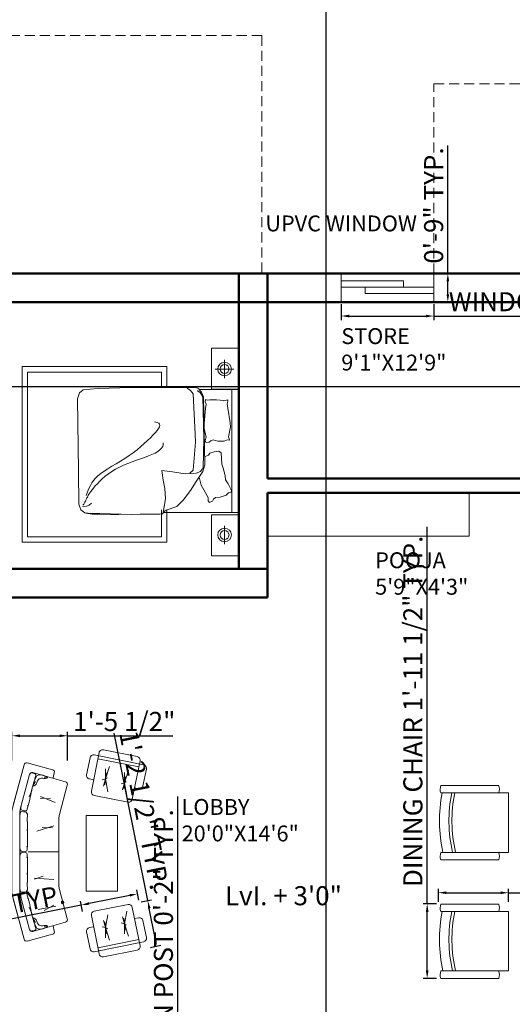
# Model space of a CAD drawing. Units: inches. Extents: x 2123 to 2977, y 1464 to 2698.
# Tile 7 of 10: x 2459 to 2614, y 2196 to 2506. Entities that reach past the tile are written whole.
import ezdxf

# ---------------------------------------------------------------- set-up
doc = ezdxf.new("R2010")
doc.units = ezdxf.units.IN
doc.linetypes.add('HIDDEN2', pattern=[4.7625, 3.175, -1.5875])
for name, color, linetype, lineweight in [('A-ANNO-DIMS', 2, 'Continuous', 18), ('A-ANNO-SYMB', 7, 'Continuous', 18), ('A-ANNO-TEXT', 7, 'Continuous', 18), ('A-AREA-IDEN', 7, 'Continuous', 25), ('A-FLOR-OVHD', 253, 'HIDDEN2', 18), ('A-FURN', 8, 'Continuous', 18), ('A-FURN-FIXD', 8, 'Continuous', 20), ('A-GLAZ', 4, 'Continuous', 18), ('A-WALL', 7, 'Continuous', 50)]:
    doc.layers.add(name, color=color, linetype=linetype, lineweight=lineweight)
doc.styles.get("Standard").update_dxf_attribs({"font": 'arial.ttf'})
doc.dimstyles.new('ISO-25', dxfattribs={"dimtxt": 6, "dimasz": 2.5, "dimexe": 1.25, "dimexo": 0.625, "dimtad": 1, "dimdec": 0, "dimlunit": 3, "dimtxsty": 'Standard', "dimcen": 2.5, "dimadec": 0, "dimazin": 0, "dimtfac": 1, "dimtdec": 0, "dimtmove": 0, "dimatfit": 3, "dimfxl": 1, "dimarcsym": 0})

# ---------------------------------------------------------------- blocks, each defined once
blk = doc.blocks.new('КРЕСЛО04')
for p, q in [((-70, 400), (-820, 400)), ((-760, 480), (-760, -480)), ((-700, 400), (-700, -400)), ((-690, 550), (-360, 550)), ((-290, 400), (-290, 480)), ((-890, 330), (-890, -330)), ((-350, 180), (-540, 220)), ((-350, 180), (-470, 190)), ((-350, 180), (-320, 240)), ((-350, 180), (-210, 190)), ((0, -330), (0, 330)), ((-350, 180), (-600, 150)), ((-350, 180), (-380, 150)), ((-350, 180), (-120, 90)), ((-350, 180), (-240, 170)), ((-350, -190), (-540, -150)), ((-350, -190), (-470, -180)), ((-350, -190), (-320, -130)), ((-350, -190), (-210, -180)), ((-350, -190), (-600, -220)), ((-350, -190), (-380, -220)), ((-350, -190), (-120, -280)), ((-350, -190), (-240, -200)), ((-820, -400), (-70, -400)), ((-690, -550), (-360, -550)), ((-290, -400), (-290, -480))]:
    blk.add_line(p, q)
for centre, start, end in [((-820, 330), 90, 180), ((-690, 480), 90, 180), ((-360, 480), 360, 90), ((-70, 330), 360, 90), ((-820, -330), 180, 270), ((-70, -330), 270, 360), ((-690, -480), 180, 270), ((-360, -480), 270, 360)]:
    blk.add_arc(centre, 70, start, end)
blk = doc.blocks.new('ДИВАН08')
for p, q in [((777, 1575), (294, 1705)), ((10, 838), (233, 1669)), ((233, 1669), (26, 897)), ((1026, 1343), (400, 1521)), ((812, 1514), (787, 1417)), ((339, 1486), (160, 818)), ((400, 1260), (453, 1348)), ((691, 1435), (619, 1433)), ((910, 720), (1061, 1282)), ((540, 1030), (740, 1020)), ((550, 1060), (830, 950)), ((0, 761), (0, -761)), ((150, 741), (150, -741)), ((900, 642), (900, -642)), ((480, 400), (800, 500)), ((780, 460), (580, 470)), ((310, 0), (900, 0)), ((600, -460), (430, -520)), ((430, -500), (800, -530)), ((910, -720), (1061, -1282)), ((10, -838), (233, -1669)), ((233, -1669), (26, -897)), ((339, -1486), (160, -818)), ((500, -1100), (840, -1040)), ((800, -1020), (620, -1120)), ((400, -1260), (453, -1348)), ((1026, -1343), (400, -1521)), ((691, -1435), (619, -1433)), ((812, -1514), (787, -1417)), ((777, -1575), (294, -1705))]:
    blk.add_line(p, q)
for centre, radius, start, end in [((281, 1656), 50, 75, 165), ((387, 1473), 50, 75, 165), ((362, 1495), 20, 89.0297, 94.7193), ((359, 1330), 185, 60.9703, 89.0297), ((764, 1527), 50, 345, 75), ((439, 1474), 20, 345, 60.9703), ((1013, 1295), 50, 345, 75), ((-610, 1509), 1045, 334.4223, 341.4421), ((298, 1228), 90.2, 326.9449, 350.757), ((300, 761), 300, 165, 180), ((450, 741), 300, 165, 180), ((242, 847), 72.2, 156.1517, 210.7358), ((269, 972), 185, 240.9703, 269.0297), ((266, 807), 20, 269.0297, 345), ((213, 880), 92.8, 338.027, 9.0149), ((-57, 544), 353, 1.9165, 10.4824), ((1200, 642), 300, 165, 180), ((-23, 353), 322, 358.4137, 13.7556), ((86, 55), 209, 1.7155, 15.9571), ((86, -55), 209, 344.0429, 358.2845), ((-23, -353), 322, 346.2444, 1.5863), ((-57, -544), 353, 349.5176, 358.0835), ((450, -741), 300, 180, 195), ((1200, -642), 300, 180, 195), ((300, -761), 300, 180, 195), ((242, -847), 72.2, 149.2642, 203.8483), ((269, -972), 185, 90.9703, 119.0297), ((266, -807), 20, 15, 90.9703), ((213, -880), 92.8, 350.9851, 21.973), ((-610, -1509), 1045, 18.5579, 25.5777), ((298, -1228), 90.2, 9.243, 33.0551), ((1013, -1295), 50, 285, 15), ((387, -1473), 50, 195, 285), ((359, -1330), 185, 270.9703, 299.0297), ((439, -1474), 20, 299.0297, 15), ((281, -1656), 50, 195, 285), ((362, -1495), 20, 265.2807, 270.9703), ((764, -1527), 50, 285, 15)]:
    blk.add_arc(centre, radius, start, end)
for points, knots in [([(459, 1469), (452, 1440), (431, 1359), (378, 1199), (347, 1000), (304, 860), (286, 801)], [0, 0, 0, 0, 90.187713, 250.973361, 505.38742, 689.989893, 689.989893, 689.989893, 689.989893]), ([(398, 1251), (413, 1308), (433, 1384), (489, 1480), (588, 1481), (651, 1453), (691, 1435)], [0, 0, 0, 0, 182.307841, 236.159489, 312.31722, 446.240501, 446.240501, 446.240501, 446.240501]), ([(400, 1260), (417, 1265), (477, 1281), (481, 1367), (520, 1397), (525, 1401)], [0, 0, 0, 0, 50, 176.134878, 196.761653, 196.761653, 196.761653, 196.761653]), ([(525, 1401), (539, 1407), (583, 1425), (652, 1391), (683, 1425), (691, 1435)], [0, 0, 0, 0, 44.660676, 140.870988, 176.926501, 176.926501, 176.926501, 176.926501]), ([(156, 55), (155, 68), (151, 132), (151, 244), (150, 392), (154, 520), (148, 633), (153, 704), (162, 778), (223, 769), (278, 775), (303, 714), (290, 642), (303, 516), (300, 345), (298, 186), (295, 82), (296, 27), (255, 6), (217, 1), (173, 12), (157, 41), (156, 55)], [0, 0, 0, 0, 37.52683, 194.502639, 336.34661, 480.520736, 579.37384, 668.990026, 713.725273, 764.098689, 821.099919, 865.09763, 933.523372, 1043.042771, 1240.322997, 1451.300934, 1509.736774, 1565.888367, 1594.82446, 1636.840587, 1680.06496, 1722.682399, 1722.682399, 1722.682399, 1722.682399]), ([(156, -55), (155, -68), (151, -132), (151, -244), (150, -392), (154, -520), (148, -633), (153, -704), (162, -778), (223, -769), (278, -775), (303, -714), (290, -642), (303, -516), (300, -345), (298, -186), (295, -82), (296, -27), (255, -6), (217, -1), (173, -12), (157, -41), (156, -55)], [0, 0, 0, 0, 37.52683, 194.502639, 336.34661, 480.520736, 579.37384, 668.990026, 713.725273, 764.098689, 821.099919, 865.09763, 933.523372, 1043.042771, 1240.322997, 1451.300934, 1509.736774, 1565.888367, 1594.82446, 1636.840587, 1680.06496, 1722.682399, 1722.682399, 1722.682399, 1722.682399]), ([(459, -1469), (452, -1440), (431, -1359), (378, -1199), (347, -1000), (304, -860), (286, -801)], [0, 0, 0, 0, 90.187713, 250.973361, 505.38742, 689.989893, 689.989893, 689.989893, 689.989893]), ([(398, -1251), (413, -1308), (433, -1384), (489, -1480), (588, -1481), (651, -1453), (691, -1435)], [0, 0, 0, 0, 182.307841, 236.159489, 312.31722, 446.240501, 446.240501, 446.240501, 446.240501]), ([(400, -1260), (417, -1265), (477, -1281), (481, -1367), (520, -1397), (525, -1401)], [0, 0, 0, 0, 50, 176.134878, 196.761653, 196.761653, 196.761653, 196.761653]), ([(525, -1401), (539, -1407), (583, -1425), (652, -1391), (683, -1425), (691, -1435)], [0, 0, 0, 0, 44.660676, 140.870988, 176.926501, 176.926501, 176.926501, 176.926501])]:
    blk.add_open_spline(points, degree=3, knots=knots)
blk = doc.blocks.new('DINING-CHAIR')
for p, q in [((0.42, 23.4), (18.64, 23.4)), ((0.39, 21.06), (21.73, 21.06)), ((21.73, 21.06), (21.73, 2.34)), ((18.66, 0), (0.38, 0)), ((21.73, 2.34), (0.43, 2.34))]:
    blk.add_line(p, q)
for centre, radius, start, end in [((3.85, 22.18), 3.64, 160.4535, 197.9116), ((15.19, 22.21), 3.64, 342.2774, 19.7376), ((46.03, 12.27), 46.04, 168.9982, 192.4562), ((46.66, 12.27), 43.7, 168.4012, 193.1346), ((46.66, 12.27), 42.76, 168.1438, 193.4274), ((3.85, 1.11), 3.64, 160.2624, 197.7226), ((15.19, 1.11), 3.64, 342.2774, 19.7376)]:
    blk.add_arc(centre, radius, start, end)
blk = doc.blocks.new('WINDOW-UPVC-29')
for p, q in [((0, 4.7), (0, 9)), ((0, 9), (0, 0)), ((19.61, 6.7), (0, 6.7)), ((19.61, 6.7), (19.61, 4.7)), ((29.17, 9), (29.17, 0)), ((29.17, 4.7), (0, 4.7)), ((7.53, 2.7), (7.53, 4.7)), ((29.17, 2.7), (7.53, 2.7))]:
    blk.add_line(p, q)
blk = doc.blocks.new('*D22')
at = {"layer": 'A-ANNO-DIMS', "color": 0, "lineweight": -2, "transparency": 16777216}
for p, q in [((2509.18, 2158.53), (2509.18, 2261.23)), ((2509.18, 2154.01), (2509.18, 2156.03)), ((2509.5, 2156.03), (2510.43, 2156.03)), ((2509.18, 2151.51), (2509.18, 2149.01)), ((2509.5, 2154.01), (2510.43, 2154.01))]:
    blk.add_line(p, q, dxfattribs=at)
at = {"layer": 'A-ANNO-DIMS', "color": 0, "transparency": 16777216}
for points in [[(2508.76, 2158.53), (2509.6, 2158.53), (2509.18, 2156.03)], [(2508.76, 2151.51), (2509.6, 2151.51), (2509.18, 2154.01)]]:
    blk.add_solid(points, dxfattribs=at)
at = {"layer": 'Defpoints', "color": 0, "transparency": 16777216}
for p in [(2508.88, 2156.03), (2509.18, 2156.03), (2508.88, 2154.01)]:
    blk.add_point(p, dxfattribs=at)
at = {"layer": 'A-ANNO-DIMS', "color": 0, "transparency": 16777216, "insert": (2505.45, 2211.13), "char_height": 6, "attachment_point": 5, "rotation": 90}
blk.add_mtext('SCREEN POST 0\'-2" TYP.', dxfattribs=at)
blk = doc.blocks.new('*D31')
at = {"layer": 'A-ANNO-DIMS', "color": 0, "lineweight": -2, "transparency": 16777216}
for p, q in [((2456.99, 2272.54), (2456.99, 2281.61)), ((2474.54, 2272.54), (2474.54, 2281.61)), ((2459.49, 2280.36), (2472.04, 2280.36)), ((2474.54, 2280.36), (2507.66, 2280.36))]:
    blk.add_line(p, q, dxfattribs=at)
at = {"layer": 'A-ANNO-DIMS', "color": 0, "transparency": 16777216}
for points in [[(2459.49, 2280.77), (2459.49, 2279.94), (2456.99, 2280.36)], [(2472.04, 2280.77), (2472.04, 2279.94), (2474.54, 2280.36)]]:
    blk.add_solid(points, dxfattribs=at)
at = {"layer": 'Defpoints', "color": 0, "transparency": 16777216}
for p in [(2474.54, 2280.36), (2456.99, 2271.92), (2474.54, 2271.92)]:
    blk.add_point(p, dxfattribs=at)
at = {"layer": 'A-ANNO-DIMS', "color": 0, "transparency": 16777216, "insert": (2492.35, 2284.08), "char_height": 6, "attachment_point": 5}
blk.add_mtext('1\'-5 1/2"', dxfattribs=at)
blk = doc.blocks.new('*D32')
at = {"layer": 'A-ANNO-DIMS', "color": 0, "lineweight": -2, "transparency": 16777216}
for p, q in [((2496.96, 2228.58), (2496.31, 2231.85)), ((2494.1, 2230.13), (2481.27, 2227.57)), ((2478.82, 2227.08), (2411.5, 2213.61)), ((2479.23, 2225.03), (2478.58, 2228.3))]:
    blk.add_line(p, q, dxfattribs=at)
at = {"layer": 'A-ANNO-DIMS', "color": 0, "transparency": 16777216}
for points in [[(2494.02, 2230.54), (2494.18, 2229.73), (2496.55, 2230.62)], [(2481.19, 2227.98), (2481.36, 2227.16), (2478.82, 2227.08)]]:
    blk.add_solid(points, dxfattribs=at)
at = {"layer": 'Defpoints', "color": 0, "transparency": 16777216}
for p in [(2478.82, 2227.08), (2497.08, 2227.96), (2479.36, 2224.42)]:
    blk.add_point(p, dxfattribs=at)
at = {"layer": 'A-ANNO-DIMS', "color": 0, "transparency": 16777216, "insert": (2443.2, 2223.76), "char_height": 6, "attachment_point": 5, "rotation": 11.3099}
blk.add_mtext('CHAIR 1\'-6" TYP.', dxfattribs=at)
blk = doc.blocks.new('*D33')
at = {"layer": 'A-ANNO-DIMS', "color": 0, "lineweight": -2, "transparency": 16777216}
for p, q in [((2499.74, 2228.5), (2489.2, 2281.19)), ((2497.7, 2228.09), (2500.97, 2228.74)), ((2502.12, 2216.6), (2500.23, 2226.04)), ((2500.57, 2213.74), (2503.84, 2214.4))]:
    blk.add_line(p, q, dxfattribs=at)
at = {"layer": 'A-ANNO-DIMS', "color": 0, "transparency": 16777216}
for points in [[(2500.64, 2226.13), (2499.83, 2225.96), (2499.74, 2228.5)], [(2502.53, 2216.69), (2501.71, 2216.52), (2502.61, 2214.15)]]:
    blk.add_solid(points, dxfattribs=at)
at = {"layer": 'Defpoints', "color": 0, "transparency": 16777216}
for p in [(2497.08, 2227.96), (2499.74, 2228.5), (2499.95, 2213.62)]:
    blk.add_point(p, dxfattribs=at)
at = {"layer": 'A-ANNO-DIMS', "color": 0, "transparency": 16777216, "insert": (2497.88, 2256.8), "char_height": 6, "attachment_point": 5, "rotation": 281.3099}
blk.add_mtext('1\'-2 1/2" TYP.', dxfattribs=at)
blk = doc.blocks.new('*D34')
at = {"layer": 'A-ANNO-DIMS', "color": 0, "lineweight": -2, "transparency": 16777216}
for p, q in [((2587.69, 2227.43), (2587.69, 2346.17)), ((2590.58, 2227.43), (2586.44, 2227.43)), ((2587.69, 2206.49), (2587.69, 2224.93)), ((2590.58, 2203.99), (2586.44, 2203.99))]:
    blk.add_line(p, q, dxfattribs=at)
at = {"layer": 'A-ANNO-DIMS', "color": 0, "transparency": 16777216}
for points in [[(2587.27, 2224.93), (2588.11, 2224.93), (2587.69, 2227.43)], [(2587.27, 2206.49), (2588.11, 2206.49), (2587.69, 2203.99)]]:
    blk.add_solid(points, dxfattribs=at)
at = {"layer": 'Defpoints', "color": 0, "transparency": 16777216}
for p in [(2587.69, 2227.43), (2591.21, 2227.43), (2591.21, 2203.99)]:
    blk.add_point(p, dxfattribs=at)
at = {"layer": 'A-ANNO-DIMS', "color": 0, "transparency": 16777216, "insert": (2583.96, 2288.05), "char_height": 6, "attachment_point": 5, "rotation": 90}
blk.add_mtext('DINING CHAIR 1\'-11 1/2" TYP.', dxfattribs=at)
blk = doc.blocks.new('*D35')
at = {"layer": 'A-ANNO-DIMS', "color": 0, "lineweight": -2, "transparency": 16777216}
for p, q in [((2591.21, 2228.06), (2591.21, 2232.2)), ((2613.29, 2228.06), (2613.29, 2232.2)), ((2593.71, 2230.95), (2610.79, 2230.95)), ((2613.29, 2230.95), (2657.71, 2230.95))]:
    blk.add_line(p, q, dxfattribs=at)
at = {"layer": 'A-ANNO-DIMS', "color": 0, "transparency": 16777216}
for points in [[(2593.71, 2231.37), (2593.71, 2230.53), (2591.21, 2230.95)], [(2610.79, 2231.37), (2610.79, 2230.53), (2613.29, 2230.95)]]:
    blk.add_solid(points, dxfattribs=at)
at = {"layer": 'Defpoints', "color": 0, "transparency": 16777216}
for p in [(2613.29, 2230.95), (2591.21, 2227.43), (2613.29, 2227.43)]:
    blk.add_point(p, dxfattribs=at)
at = {"layer": 'A-ANNO-DIMS', "color": 0, "transparency": 16777216, "insert": (2636.75, 2234.64), "char_height": 6, "attachment_point": 5}
blk.add_mtext('1\'-10" TYP.', dxfattribs=at)
blk = doc.blocks.new('*D46')
at = {"layer": 'A-ANNO-DIMS', "color": 0, "lineweight": -2, "transparency": 16777216}
for p, q in [((2560.64, 2416.25), (2560.64, 2411.24)), ((2589.82, 2416.25), (2589.82, 2411.24)), ((2563.14, 2412.49), (2587.32, 2412.49)), ((2589.82, 2412.49), (2669.49, 2412.49))]:
    blk.add_line(p, q, dxfattribs=at)
at = {"layer": 'A-ANNO-DIMS', "color": 0, "transparency": 16777216}
for points in [[(2563.14, 2412.91), (2563.14, 2412.08), (2560.64, 2412.49)], [(2587.32, 2412.91), (2587.32, 2412.08), (2589.82, 2412.49)]]:
    blk.add_solid(points, dxfattribs=at)
at = {"layer": 'Defpoints', "color": 0, "transparency": 16777216}
for p in [(2560.64, 2416.87), (2589.82, 2416.87), (2589.82, 2412.49)]:
    blk.add_point(p, dxfattribs=at)
at = {"layer": 'A-ANNO-DIMS', "color": 0, "transparency": 16777216, "insert": (2630.9, 2416.22), "char_height": 6, "attachment_point": 5}
blk.add_mtext('WINDOW 2\'-5" TYP.', dxfattribs=at)
blk = doc.blocks.new('*D47')
at = {"layer": 'A-ANNO-DIMS', "color": 0, "lineweight": -2, "transparency": 16777216}
for p, q in [((2594.19, 2425.87), (2594.19, 2466.19)), ((2590.44, 2425.87), (2595.44, 2425.87)), ((2594.19, 2419.37), (2594.19, 2423.37)), ((2590.44, 2416.87), (2595.44, 2416.87))]:
    blk.add_line(p, q, dxfattribs=at)
at = {"layer": 'A-ANNO-DIMS', "color": 0, "transparency": 16777216}
for points in [[(2593.78, 2423.37), (2594.61, 2423.37), (2594.19, 2425.87)], [(2593.78, 2419.37), (2594.61, 2419.37), (2594.19, 2416.87)]]:
    blk.add_solid(points, dxfattribs=at)
at = {"layer": 'Defpoints', "color": 0, "transparency": 16777216}
for p in [(2589.82, 2425.87), (2594.19, 2425.87), (2589.82, 2416.87)]:
    blk.add_point(p, dxfattribs=at)
at = {"layer": 'A-ANNO-DIMS', "color": 0, "transparency": 16777216, "insert": (2590.5, 2447.28), "char_height": 6, "attachment_point": 5, "rotation": 90}
blk.add_mtext('0\'-9" TYP.', dxfattribs=at)
blk = doc.blocks.new('*D57')
at = {"layer": 'A-ANNO-DIMS', "color": 0, "lineweight": -2, "transparency": 16777216}
for p, q in [((2555.89, 1805.13), (2555.89, 2606.82)), ((2757.94, 1805.13), (2757.94, 2606.82)), ((2558.39, 2605.57), (2755.44, 2605.57))]:
    blk.add_line(p, q, dxfattribs=at)
at = {"layer": 'A-ANNO-DIMS', "color": 0, "transparency": 16777216}
for points in [[(2558.39, 2605.99), (2558.39, 2605.15), (2555.89, 2605.57)], [(2755.44, 2605.99), (2755.44, 2605.15), (2757.94, 2605.57)]]:
    blk.add_solid(points, dxfattribs=at)
at = {"layer": 'Defpoints', "color": 0, "transparency": 16777216}
for p in [(2757.94, 2605.57), (2555.89, 1804.5), (2757.94, 1804.5)]:
    blk.add_point(p, dxfattribs=at)
at = {"layer": 'A-ANNO-DIMS', "color": 0, "transparency": 16777216, "insert": (2656.91, 2609.26), "char_height": 6, "attachment_point": 5}
blk.add_mtext('16\'-10"', dxfattribs=at)
blk = doc.blocks.new('*D59')
at = {"layer": 'A-ANNO-DIMS', "color": 0, "lineweight": -2, "transparency": 16777216}
for p, q in [((2819.64, 2416.87), (2819.64, 2450.65)), ((2376.14, 2416.87), (2820.89, 2416.87)), ((2819.64, 2392.84), (2819.64, 2414.37)), ((2344.56, 2390.34), (2820.89, 2390.34))]:
    blk.add_line(p, q, dxfattribs=at)
at = {"layer": 'A-ANNO-DIMS', "color": 0, "transparency": 16777216}
for points in [[(2819.22, 2414.37), (2820.05, 2414.37), (2819.64, 2416.87)], [(2819.22, 2392.84), (2820.05, 2392.84), (2819.64, 2390.34)]]:
    blk.add_solid(points, dxfattribs=at)
at = {"layer": 'Defpoints', "color": 0, "transparency": 16777216}
for p in [(2375.52, 2416.87), (2819.64, 2416.87), (2343.94, 2390.34)]:
    blk.add_point(p, dxfattribs=at)
at = {"layer": 'A-ANNO-DIMS', "color": 0, "transparency": 16777216, "insert": (2815.91, 2435.01), "char_height": 6, "attachment_point": 5, "rotation": 90}
blk.add_mtext('2\'-2 1/2"', dxfattribs=at)

msp = doc.modelspace()

# ---------------------------------------------------------------- linework, layer by layer
at = {"layer": 'A-FLOR-OVHD'}
for p, q in [((2332.44, 2500.76), (2535.66, 2500.76)), ((2535.66, 2500.76), (2535.66, 2425.87)), ((2589.82, 2425.87), (2589.82, 2485.57)), ((2589.82, 2485.57), (2757.94, 2485.57)), ((2589.82, 2425.87), (2589.82, 2425.87))]:
    msp.add_line(p, q, dxfattribs=at)
at = {"layer": 'A-FURN'}
for p, q in [((2523.94, 2398.74), (2523.94, 2392.88)), ((2523.94, 2398.74), (2523.94, 2392.88)), ((2526.87, 2395.81), (2521.01, 2395.81)), ((2526.87, 2395.81), (2521.01, 2395.81)), ((2494.31, 2390.03), (2484.25, 2389.63)), ((2494.31, 2390.03), (2484.25, 2389.63)), ((2513.07, 2389.95), (2494.31, 2390.03)), ((2513.07, 2389.95), (2494.31, 2390.03)), ((2514.48, 2389.98), (2513.07, 2389.95)), ((2514.48, 2389.98), (2513.07, 2389.95)), ((2515.08, 2389.92), (2514.48, 2389.98)), ((2515.08, 2389.92), (2514.48, 2389.98)), ((2478.3, 2388.31), (2477.68, 2386.47)), ((2478.3, 2388.31), (2477.68, 2386.47)), ((2479.45, 2389.25), (2478.3, 2388.31)), ((2479.45, 2389.25), (2478.3, 2388.31)), ((2481.62, 2389.49), (2479.45, 2389.25)), ((2481.62, 2389.49), (2479.45, 2389.25)), ((2484.25, 2389.63), (2481.62, 2389.49)), ((2484.25, 2389.63), (2481.62, 2389.49)), ((2515.94, 2389.37), (2528.4, 2389.37)), ((2515.94, 2389.37), (2528.4, 2389.37)), ((2477.93, 2363.85), (2477.68, 2386.47)), ((2477.93, 2363.85), (2477.68, 2386.47)), ((2523.66, 2385.81), (2524.91, 2386.14)), ((2523.66, 2385.81), (2524.91, 2386.14)), ((2518.17, 2374.33), (2517.37, 2377.47)), ((2518.17, 2374.33), (2517.37, 2377.47)), ((2525.13, 2374.48), (2525.79, 2377.66)), ((2525.13, 2374.48), (2525.79, 2377.66)), ((2525.79, 2377.66), (2525.66, 2378.83)), ((2525.79, 2377.66), (2525.66, 2378.83)), ((2517.86, 2373.34), (2518.17, 2374.33)), ((2517.86, 2373.34), (2518.17, 2374.33)), ((2525.49, 2373.51), (2525.13, 2374.48)), ((2525.49, 2373.51), (2525.13, 2374.48)), ((2518.06, 2372.73), (2517.86, 2373.34)), ((2518.06, 2372.73), (2517.86, 2373.34)), ((2519.09, 2372.79), (2518.06, 2372.73)), ((2519.09, 2372.79), (2518.06, 2372.73)), ((2519.65, 2373.22), (2519.09, 2372.79)), ((2519.65, 2373.22), (2519.09, 2372.79)), ((2520.36, 2373.47), (2519.65, 2373.22)), ((2520.36, 2373.47), (2519.65, 2373.22)), ((2521.82, 2373.11), (2520.36, 2373.47)), ((2521.82, 2373.11), (2520.36, 2373.47)), ((2523.8, 2373.1), (2521.82, 2373.11)), ((2523.8, 2373.1), (2521.82, 2373.11)), ((2524.74, 2373.49), (2523.8, 2373.1)), ((2524.74, 2373.49), (2523.8, 2373.1)), ((2525.46, 2373.41), (2524.74, 2373.49)), ((2525.46, 2373.41), (2524.74, 2373.49)), ((2525.46, 2373.41), (2524.74, 2373.49)), ((2525.46, 2373.41), (2524.74, 2373.49)), ((2525.46, 2373.41), (2525.49, 2373.51)), ((2525.46, 2373.41), (2525.49, 2373.51)), ((2522.83, 2369.47), (2523.05, 2365.83)), ((2522.83, 2369.47), (2523.05, 2365.83)), ((2523.05, 2365.83), (2523.51, 2364.59)), ((2523.05, 2365.83), (2523.51, 2364.59)), ((2477.93, 2363.85), (2477.93, 2359.23)), ((2477.93, 2363.85), (2477.93, 2359.23)), ((2523.51, 2364.59), (2524.14, 2362.26)), ((2523.51, 2364.59), (2524.14, 2362.26)), ((2524.14, 2362.26), (2524.25, 2360.9)), ((2524.14, 2362.26), (2524.25, 2360.9)), ((2477.93, 2359.23), (2478.05, 2357.59)), ((2477.93, 2359.23), (2478.05, 2357.59)), ((2518.72, 2355.39), (2516.58, 2359.21)), ((2518.72, 2355.39), (2516.58, 2359.21)), ((2524.25, 2360.9), (2525.06, 2359.69)), ((2524.25, 2360.9), (2525.06, 2359.69)), ((2524.25, 2360.9), (2525.06, 2359.69)), ((2524.25, 2360.9), (2525.06, 2359.69)), ((2525.06, 2359.69), (2525.85, 2357.98)), ((2525.06, 2359.69), (2525.85, 2357.98)), ((2478.05, 2357.59), (2478.05, 2353.27)), ((2478.05, 2357.59), (2478.05, 2353.27)), ((2524.43, 2356.14), (2522.57, 2355.48)), ((2524.43, 2356.14), (2522.57, 2355.48)), ((2525.18, 2356.82), (2524.43, 2356.14)), ((2525.18, 2356.82), (2524.43, 2356.14)), ((2478.72, 2351.46), (2478.05, 2353.27)), ((2478.72, 2351.46), (2478.05, 2353.27)), ((2479.17, 2352.58), (2480.45, 2352.64)), ((2479.17, 2352.58), (2480.45, 2352.64)), ((2480.45, 2352.64), (2481.33, 2352.93)), ((2480.45, 2352.64), (2481.33, 2352.93)), ((2481.33, 2352.93), (2481.99, 2353.56)), ((2481.33, 2352.93), (2481.99, 2353.56)), ((2518.76, 2354.35), (2518.72, 2355.39)), ((2518.76, 2354.35), (2518.72, 2355.39)), ((2519.15, 2353.84), (2518.76, 2354.35)), ((2519.15, 2353.84), (2518.76, 2354.35)), ((2520.11, 2354.25), (2519.15, 2353.84)), ((2520.11, 2354.25), (2519.15, 2353.84)), ((2520.49, 2354.85), (2520.11, 2354.25)), ((2520.49, 2354.85), (2520.11, 2354.25)), ((2521.07, 2355.32), (2520.49, 2354.85)), ((2521.07, 2355.32), (2520.49, 2354.85)), ((2522.57, 2355.48), (2521.07, 2355.32)), ((2522.57, 2355.48), (2521.07, 2355.32)), ((2479.9, 2350.54), (2478.72, 2351.46)), ((2479.9, 2350.54), (2478.72, 2351.46)), ((2482.07, 2350.37), (2479.9, 2350.54)), ((2482.07, 2350.37), (2479.9, 2350.54)), ((2480.3, 2350.43), (2482.22, 2350.07)), ((2480.3, 2350.43), (2482.22, 2350.07)), ((2484.71, 2350.31), (2482.07, 2350.37)), ((2484.71, 2350.31), (2482.07, 2350.37)), ((2482.22, 2350.07), (2484.07, 2349.96)), ((2482.22, 2350.07), (2484.07, 2349.96)), ((2484.07, 2349.96), (2497.39, 2350.1)), ((2484.07, 2349.96), (2497.39, 2350.1)), ((2494.78, 2350.05), (2484.71, 2350.31)), ((2494.78, 2350.05), (2484.71, 2350.31)), ((2497.39, 2350.1), (2503.48, 2350.16)), ((2497.39, 2350.1), (2503.48, 2350.16)), ((2504.61, 2350.67), (2504.65, 2350.59)), ((2504.61, 2350.67), (2504.65, 2350.59)), ((2523.94, 2340.64), (2523.94, 2346.5)), ((2523.94, 2340.64), (2523.94, 2346.5)), ((2480.33, 2231.45), (2480.33, 2255.28)), ((2480.33, 2255.28), (2490.19, 2255.28)), ((2490.19, 2255.28), (2490.19, 2231.45)), ((2490.19, 2231.45), (2480.33, 2231.45))]:
    msp.add_line(p, q, dxfattribs=at)
for points in [[(2519.78, 2402.34), (2519.78, 2389.42), (2528.39, 2389.42), (2528.39, 2402.34)], [(2519.78, 2402.34), (2519.78, 2389.42), (2528.39, 2389.42), (2528.39, 2402.34)], [(2519.78, 2337.05), (2519.78, 2349.96), (2528.39, 2349.96), (2528.39, 2337.05)], [(2519.78, 2337.05), (2519.78, 2349.96), (2528.39, 2349.96), (2528.39, 2337.05)]]:
    msp.add_lwpolyline(points, close=True, dxfattribs=at)
for points in [[(2505.75, 2351.44), (2505.75, 2341.3), (2460.23, 2341.3), (2460.23, 2396.57), (2505.75, 2396.57), (2505.75, 2389.99)], [(2505.75, 2351.44), (2505.75, 2341.3), (2460.23, 2341.3), (2460.23, 2396.57), (2505.75, 2396.57), (2505.75, 2389.99)], [(2504.03, 2351.44), (2504.03, 2343.03), (2461.95, 2343.03), (2461.95, 2394.85), (2504.03, 2394.85), (2504.03, 2389.99)], [(2504.03, 2351.44), (2504.03, 2343.03), (2461.95, 2343.03), (2461.95, 2394.85), (2504.03, 2394.85), (2504.03, 2389.99)], [(2513.04, 2363.03), (2514.04, 2364), (2514.78, 2372.74), (2514.63, 2375.29), (2513.99, 2387.95), (2513.19, 2389.02), (2512.11, 2389.82)], [(2513.04, 2363.03), (2514.04, 2364), (2514.78, 2372.74), (2514.63, 2375.29), (2513.99, 2387.95), (2513.19, 2389.02), (2512.11, 2389.82)], [(2515.12, 2389.9), (2515.52, 2389.78), (2515.83, 2389.59), (2515.94, 2389.37), (2516.16, 2389.12), (2516.17, 2389.08)], [(2515.12, 2389.9), (2515.52, 2389.78), (2515.83, 2389.59), (2515.94, 2389.37), (2516.16, 2389.12), (2516.17, 2389.08)], [(2504.59, 2350.6), (2505.35, 2354.95), (2505.11, 2358.16), (2504.58, 2360.78), (2504.15, 2363.88), (2507.54, 2363.46), (2511.48, 2362.77), (2514.97, 2363.07), (2516.38, 2363.53), (2517.19, 2364.67), (2517.44, 2373.85), (2517.04, 2387.06), (2516.24, 2388.41), (2515.45, 2388.98), (2515.38, 2389.06)], [(2504.59, 2350.6), (2505.35, 2354.95), (2505.11, 2358.16), (2504.58, 2360.78), (2504.15, 2363.88), (2507.54, 2363.46), (2511.48, 2362.77), (2514.97, 2363.07), (2516.38, 2363.53), (2517.19, 2364.67), (2517.44, 2373.85), (2517.04, 2387.06), (2516.24, 2388.41), (2515.45, 2388.98), (2515.38, 2389.06)], [(2516.17, 2389.05), (2516.63, 2388.51), (2517.24, 2387.06), (2517.66, 2365.65), (2517.11, 2363.5), (2514.82, 2360.06), (2513.39, 2357.89), (2511.01, 2354.65), (2508.9, 2352.57), (2505.51, 2351.35), (2504.62, 2350.75)], [(2516.17, 2389.05), (2516.63, 2388.51), (2517.24, 2387.06), (2517.66, 2365.65), (2517.11, 2363.5), (2514.82, 2360.06), (2513.39, 2357.89), (2511.01, 2354.65), (2508.9, 2352.57), (2505.51, 2351.35), (2504.62, 2350.75)], [(2528.4, 2389.37), (2528.4, 2350.61), (2504.68, 2350.61)], [(2528.4, 2389.37), (2528.4, 2350.61), (2504.68, 2350.61)], [(2526.24, 2350.61), (2526.24, 2389.37)], [(2526.24, 2350.61), (2526.24, 2389.37)], [(2517.45, 2378.65), (2517.94, 2383.37), (2518.11, 2384.73), (2517.82, 2385.53), (2517.9, 2386.19), (2518.42, 2386.01), (2519.31, 2386.12), (2521.39, 2386.15), (2523.65, 2385.85)], [(2517.45, 2378.65), (2517.94, 2383.37), (2518.11, 2384.73), (2517.82, 2385.53), (2517.9, 2386.19), (2518.42, 2386.01), (2519.31, 2386.12), (2521.39, 2386.15), (2523.65, 2385.85)], [(2525.66, 2378.83), (2524.95, 2383.52), (2524.73, 2384.88), (2524.98, 2385.69), (2524.91, 2386.14)], [(2525.66, 2378.83), (2524.95, 2383.52), (2524.73, 2384.88), (2524.98, 2385.69), (2524.91, 2386.14)], [(2480.32, 2356.02), (2480.68, 2356.85), (2481.02, 2357.65), (2481.35, 2358.43), (2481.71, 2359.19), (2482.12, 2359.94), (2482.63, 2360.68), (2483.25, 2361.42), (2484.01, 2362.16), (2484.93, 2362.9), (2486, 2363.64), (2487.18, 2364.4), (2488.45, 2365.18), (2489.78, 2365.98), (2491.14, 2366.8), (2492.51, 2367.66), (2493.85, 2368.55), (2495.15, 2369.47), (2496.39, 2370.42), (2497.56, 2371.38), (2498.65, 2372.33), (2499.66, 2373.26), (2500.58, 2374.16), (2501.39, 2375), (2502.1, 2375.77), (2502.69, 2376.47), (2503.14, 2377.08), (2503.44, 2377.62), (2503.56, 2378.07), (2503.49, 2378.45), (2503.2, 2378.76), (2502.68, 2378.99), (2501.91, 2379.14)], [(2480.32, 2356.02), (2480.68, 2356.85), (2481.02, 2357.65), (2481.35, 2358.43), (2481.71, 2359.19), (2482.12, 2359.94), (2482.63, 2360.68), (2483.25, 2361.42), (2484.01, 2362.16), (2484.93, 2362.9), (2486, 2363.64), (2487.18, 2364.4), (2488.45, 2365.18), (2489.78, 2365.98), (2491.14, 2366.8), (2492.51, 2367.66), (2493.85, 2368.55), (2495.15, 2369.47), (2496.39, 2370.42), (2497.56, 2371.38), (2498.65, 2372.33), (2499.66, 2373.26), (2500.58, 2374.16), (2501.39, 2375), (2502.1, 2375.77), (2502.69, 2376.47), (2503.14, 2377.08), (2503.44, 2377.62), (2503.56, 2378.07), (2503.49, 2378.45), (2503.2, 2378.76), (2502.68, 2378.99), (2501.91, 2379.14)], [(2479.31, 2352.96), (2479.58, 2353.32), (2479.81, 2353.65), (2479.99, 2353.95), (2480.15, 2354.22), (2480.28, 2354.48), (2480.4, 2354.73), (2480.51, 2354.98), (2480.62, 2355.23), (2480.74, 2355.49), (2480.87, 2355.77), (2481.04, 2356.08), (2481.25, 2356.42), (2481.51, 2356.81), (2481.83, 2357.25), (2482.21, 2357.76), (2482.68, 2358.34), (2483.24, 2358.99), (2483.88, 2359.71), (2484.62, 2360.47), (2485.44, 2361.25), (2486.35, 2362.05), (2487.35, 2362.83), (2488.43, 2363.59), (2489.59, 2364.3), (2490.83, 2364.95), (2492.14, 2365.54), (2493.48, 2366.09), (2494.84, 2366.6), (2496.19, 2367.08), (2497.51, 2367.54), (2498.77, 2368), (2499.97, 2368.45), (2501.06, 2368.9), (2502.04, 2369.37), (2502.89, 2369.85), (2503.59, 2370.35), (2504.12, 2370.86), (2504.48, 2371.4), (2504.63, 2371.96), (2504.56, 2372.55)], [(2479.31, 2352.96), (2479.58, 2353.32), (2479.81, 2353.65), (2479.99, 2353.95), (2480.15, 2354.22), (2480.28, 2354.48), (2480.4, 2354.73), (2480.51, 2354.98), (2480.62, 2355.23), (2480.74, 2355.49), (2480.87, 2355.77), (2481.04, 2356.08), (2481.25, 2356.42), (2481.51, 2356.81), (2481.83, 2357.25), (2482.21, 2357.76), (2482.68, 2358.34), (2483.24, 2358.99), (2483.88, 2359.71), (2484.62, 2360.47), (2485.44, 2361.25), (2486.35, 2362.05), (2487.35, 2362.83), (2488.43, 2363.59), (2489.59, 2364.3), (2490.83, 2364.95), (2492.14, 2365.54), (2493.48, 2366.09), (2494.84, 2366.6), (2496.19, 2367.08), (2497.51, 2367.54), (2498.77, 2368), (2499.97, 2368.45), (2501.06, 2368.9), (2502.04, 2369.37), (2502.89, 2369.85), (2503.59, 2370.35), (2504.12, 2370.86), (2504.48, 2371.4), (2504.63, 2371.96), (2504.56, 2372.55)], [(2522.83, 2369.47), (2522.12, 2369.97), (2520.62, 2369.73), (2519.3, 2369.37), (2518.88, 2368.65), (2517.81, 2368.23), (2517.61, 2368.23)], [(2522.83, 2369.47), (2522.12, 2369.97), (2520.62, 2369.73), (2519.3, 2369.37), (2518.88, 2368.65), (2517.81, 2368.23), (2517.61, 2368.23)], [(2516.58, 2359.21), (2515.95, 2361.76)], [(2516.58, 2359.21), (2515.95, 2361.76)], [(2525.18, 2356.82), (2525.98, 2357.07), (2526.14, 2357.58), (2525.85, 2357.98)], [(2525.18, 2356.82), (2525.98, 2357.07), (2526.14, 2357.58), (2525.85, 2357.98)], [(2503.54, 2350.16), (2504.38, 2350.22), (2504.63, 2350.46), (2504.68, 2350.61)], [(2503.54, 2350.16), (2504.38, 2350.22), (2504.63, 2350.46), (2504.68, 2350.61)]]:
    msp.add_lwpolyline(points, dxfattribs=at)
for centre, radius in [((2523.94, 2395.81), 2.15), ((2523.94, 2395.81), 2.15), ((2523.94, 2395.81), 1.38), ((2523.94, 2395.81), 1.38), ((2523.94, 2343.57), 2.15), ((2523.94, 2343.57), 2.15), ((2523.94, 2343.57), 1.38), ((2523.94, 2343.57), 1.38)]:
    msp.add_circle(centre, radius, dxfattribs=at)
at = {"layer": 'A-FURN-FIXD'}
msp.add_lwpolyline([(2537.44, 2356.87), (2600.92, 2356.87), (2600.92, 2343.22), (2537.44, 2343.22)], close=True, dxfattribs=at)
at = {"layer": 'A-WALL'}
for p, q in [((2250.94, 2425.87), (2766.94, 2425.87)), ((2528.44, 2425.87), (2528.44, 2332.87)), ((2528.44, 2425.87), (2528.44, 2332.87)), ((2537.44, 2425.87), (2537.44, 2361.37)), ((2250.94, 2416.87), (2687.94, 2416.87)), ((2537.44, 2361.37), (2626.06, 2361.37)), ((2537.44, 2356.87), (2685.94, 2356.87)), ((2537.44, 2356.87), (2537.44, 2323.87)), ((2432.9, 2332.87), (2537.44, 2332.87)), ((2259.94, 2323.87), (2537.44, 2323.87))]:
    msp.add_line(p, q, dxfattribs=at)

# ---------------------------------------------------------------- block references
at = {"layer": 'A-FURN', "yscale": 0.0164364890095425, "zscale": 0.0164364890095425}
for p, xscale, rotation in [((2488.22, 2260.54), -0.0164364890095425, 78.69006752728792), ((2488.22, 2226.19), 0.0164364890095425, 101.3099324727121)]:
    msp.add_blockref('КРЕСЛО04', p, dxfattribs=dict(at, xscale=xscale, rotation=rotation))
at = {"layer": 'A-FURN', "xscale": 0.0164364890095425, "yscale": 0.0164364890095425, "zscale": 0.0164364890095425}
msp.add_blockref('ДИВАН08', (2456.99, 2243.78), dxfattribs=at)
at = {"layer": 'A-FURN'}
for p in [(2591.57, 2241.33), (2591.57, 2203.99)]:
    msp.add_blockref('DINING-CHAIR', p, dxfattribs=at)
at = {"layer": 'A-GLAZ'}
msp.add_blockref('WINDOW-UPVC-29', (2560.64, 2416.87), dxfattribs=at)

# ---------------------------------------------------------------- texts
at = {"layer": 'A-ANNO-SYMB', "insert": (2524.03, 2233.01), "char_height": 6, "attachment_point": 1}
msp.add_mtext_dynamic_manual_height_columns('LvI. + 3\'0"', width=197.9054, gutter_width=12.5, heights=[0], dxfattribs=at)
at = {"layer": 'A-ANNO-TEXT', "insert": (2536.76, 2444.14), "char_height": 5, "attachment_point": 1}
msp.add_mtext_dynamic_manual_height_columns('UPVC WINDOW', width=116.1895, gutter_width=12.5, heights=[0], dxfattribs=at)
at = {"layer": 'A-AREA-IDEN', "char_height": 5, "attachment_point": 1}
for s, width, insert in [('STORE\\P9\'1"X12\'9"', 148.2395, (2560.66, 2408.67)), ('POOJA\\P5\'9"X4\'3"', 139.987, (2571.32, 2338.11)), ('LOBBY\\P20\'0"X14\'6"', 190.3877, (2510.41, 2260.45))]:
    msp.add_mtext_dynamic_manual_height_columns(s, width=width, gutter_width=12.5, heights=[0], dxfattribs=dict(at, insert=insert))

# ---------------------------------------------------------------- dimensions: what is measured, and where the dimension line sits
at = {"layer": 'A-ANNO-DIMS'}
for base, p1, p2, picture, middle in [((2757.9353, 2605.5708), (2555.8869, 1804.5032), (2757.9353, 1804.5032), '*D57', (2656.9111, 2609.2592)), ((2474.5449, 2280.3563), (2456.9906, 2271.9153), (2474.5449, 2271.9153), '*D31', (2492.3527, 2284.0836))]:
    dim = msp.add_linear_dim(base=base, p1=p1, p2=p2, dimstyle='ISO-25', override={"dimdec": 1, "dimlfac": 1, "dimrnd": 0, "dimzin": 1, "dimdsep": 46, "dimlunit": 4, "dimfrac": 2}, dxfattribs=at)
    dim.commit()
    dim.dimension.update_dxf_attribs({"geometry": picture, "text_midpoint": middle})
for base, p1, p2, angle, text, picture, middle in [((2594.19, 2425.87), (2589.82, 2416.87), (2589.82, 2425.87), 90, '<> TYP.', '*D47', (2590.5, 2447.28)), ((2587.69, 2227.43), (2591.21, 2203.99), (2591.21, 2227.43), 90, 'DINING CHAIR <> TYP.', '*D34', (2583.96, 2288.05)), ((2499.74, 2228.5), (2499.95, 2213.62), (2497.08, 2227.96), 101.3099, '<> TYP.', '*D33', (2497.88, 2256.8)), ((2509.18, 2156.03), (2508.88, 2154.01), (2508.88, 2156.03), 90, 'SCREEN POST <> TYP.', '*D22', (2505.45, 2211.13)), ((2478.82, 2227.08), (2497.08, 2227.96), (2479.36, 2224.42), 191.3099, 'CHAIR <> TYP.', '*D32', (2443.2, 2223.76))]:
    dim = msp.add_linear_dim(base=base, p1=p1, p2=p2, angle=angle, text=text, dimstyle='ISO-25', override={"dimdec": 1, "dimlfac": 1, "dimrnd": 0, "dimzin": 1, "dimdsep": 46, "dimlunit": 4, "dimfrac": 2}, dxfattribs=at)
    dim.commit()
    dim.dimension.update_dxf_attribs({"geometry": picture, "text_midpoint": middle})
dim = msp.add_linear_dim(base=(2819.64, 2416.87), p1=(2343.94, 2390.34), p2=(2375.52, 2416.87), angle=90, dimstyle='ISO-25', override={"dimdec": 1, "dimlfac": 1, "dimrnd": 0, "dimzin": 1, "dimdsep": 46, "dimlunit": 4, "dimfrac": 2}, dxfattribs=at)
dim.commit()
dim.dimension.update_dxf_attribs({"geometry": '*D59', "text_midpoint": (2815.91, 2435.01)})
for base, p1, p2, text, picture, middle in [((2589.82, 2412.49), (2560.64, 2416.87), (2589.82, 2416.87), 'WINDOW <> TYP.', '*D46', (2630.9, 2416.22)), ((2613.29, 2230.95), (2591.21, 2227.43), (2613.29, 2227.43), '<> TYP.', '*D35', (2636.75, 2234.64))]:
    dim = msp.add_linear_dim(base=base, p1=p1, p2=p2, text=text, dimstyle='ISO-25', override={"dimdec": 1, "dimlfac": 1, "dimrnd": 0, "dimzin": 1, "dimdsep": 46, "dimlunit": 4, "dimfrac": 2}, dxfattribs=at)
    dim.commit()
    dim.dimension.update_dxf_attribs({"geometry": picture, "text_midpoint": middle})

doc.saveas('drawing.dxf')
